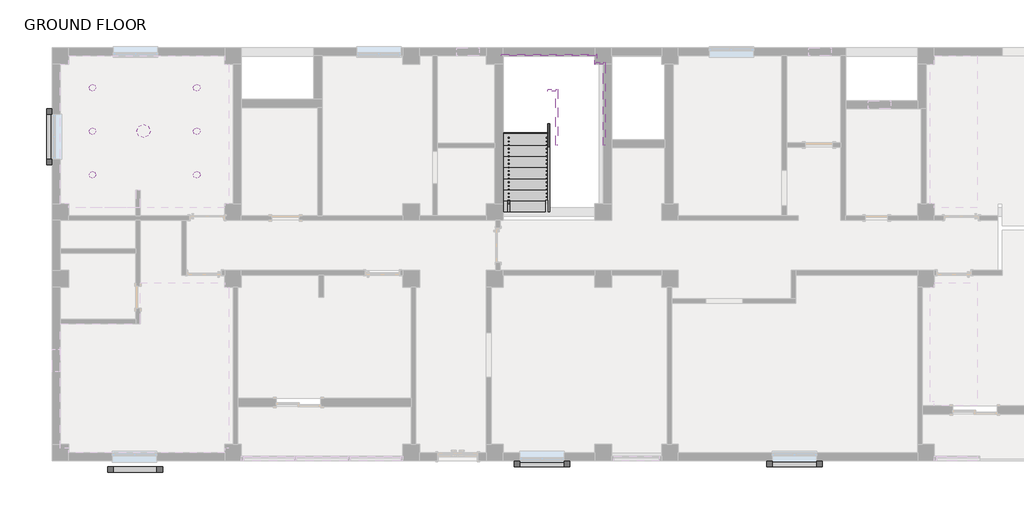
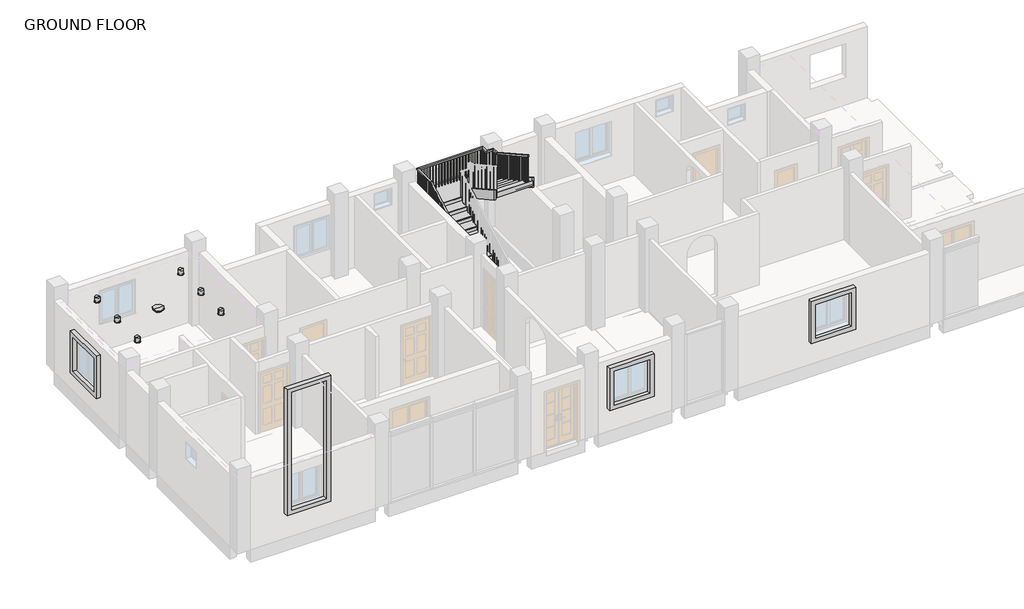
# One storey, part 5 of 5: 8 members, 7 light fixtures, 4 proxies, 1 railing, 1 stair flight.
"""IFC4 building model written with IfcOpenShell, lengths in millimetres."""

from ifc_helpers import new_model, si_unit, frame, origin, place, context, project, spatial, polyline, outline, extrude, faceted_brep, transform, mapped, element, save
from components import generic_models_17_generic_models_17_4194431e, generic_models_21_generic_models_21_07dc1754, generic_models_2_generic_models_2_798ec4a6, light_modern_pendant_14774_baffle_cc9af11b, light_modern_pendant_14774_baffle_b3430626, round_flush_mount_ceiling_light_fixture_18379_round_flush_30de1430, stair_flight_255c1e55

model = new_model("IFC4")

# Units and contexts
model_context = context("Model", 3, world=origin())
ifc_project = project(units=[si_unit("LENGTHUNIT", "METRE", prefix="MILLI")], contexts=[model_context])

# Site, building, storey
site = spatial("IfcSite", under=ifc_project)
building = spatial("IfcBuilding", under=site)
storey = spatial("IfcBuildingStorey", under=building, Name="GROUND FLOOR", Elevation=304.8)

# Proxies
placement = place(None, origin())
generic_models_17_generic_models_17_shape = generic_models_17_generic_models_17_4194431e(model_context)
element("IfcBuildingElementProxy", 1, Name="Generic Models 20 : Generic Models 17", ObjectType="Generic Models 20 : Generic Models 17", at=placement, inside=storey, context=model_context, shape_type="MappedRepresentation", body=[
    mapped(generic_models_17_generic_models_17_shape, transform((0.0, 0.0, -9144.0), x_axis=(1.0, 0.0, 0.0), y_axis=(0.0, 1.0, 0.0), z_axis=(0.0, 0.0, 1.0))),
])
generic_models_21_generic_models_21_shape = generic_models_21_generic_models_21_07dc1754(model_context)
element("IfcBuildingElementProxy", 2, Name="Generic Models 24 : Generic Models 21", ObjectType="Generic Models 24 : Generic Models 21", at=placement, inside=storey, context=model_context, shape_type="MappedRepresentation", body=[
    mapped(generic_models_21_generic_models_21_shape, transform((0.0, 0.0, -9144.0), x_axis=(1.0, 0.0, 0.0), y_axis=(0.0, 1.0, 0.0), z_axis=(0.0, 0.0, 1.0))),
])
element("IfcBuildingElementProxy", 3, Name="Generic Models 28 : Generic Models 21", ObjectType="Generic Models 28 : Generic Models 21", at=placement, inside=storey, context=model_context, shape_type="MappedRepresentation", body=[
    mapped(generic_models_21_generic_models_21_shape, transform((-6905.3372689, 0.0, -9144.0), x_axis=(1.0, 0.0, 0.0), y_axis=(0.0, 1.0, 0.0), z_axis=(0.0, 0.0, 1.0))),
])
generic_models_2_generic_models_2_shape = generic_models_2_generic_models_2_798ec4a6(model_context)
element("IfcBuildingElementProxy", 4, Name="Generic Models 3 : Generic Models 2", ObjectType="Generic Models 3 : Generic Models 2", at=placement, inside=storey, context=model_context, shape_type="MappedRepresentation", body=[
    mapped(generic_models_2_generic_models_2_shape, transform((0.0, 0.0, -6096.0), x_axis=(1.0, 0.0, 0.0), y_axis=(0.0, 1.0, 0.0), z_axis=(0.0, 0.0, 1.0))),
])

# Light fixtures
light_modern_pendant_14774_baffle_shape = light_modern_pendant_14774_baffle_cc9af11b(model_context)
element("IfcLightFixture", 5, ObjectType="LIGHT_-_MODERN_PENDANT_14774 : Baffle", at=placement, inside=storey, context=model_context, shape_type="MappedRepresentation", body=[
    mapped(light_modern_pendant_14774_baffle_shape, transform((-14269.0456086, -897.3794704, 431.8), x_axis=(1.0, 0.0, 0.0), y_axis=(0.0, 1.0, 0.0), z_axis=(0.0, 0.0, 1.0))),
])
element("IfcLightFixture", 6, ObjectType="LIGHT_-_MODERN_PENDANT_14774 : Baffle", at=placement, inside=storey, context=model_context, shape_type="MappedRepresentation", body=[
    mapped(light_modern_pendant_14774_baffle_shape, transform((-14269.0456086, -3284.9794704, 431.8), x_axis=(1.0, 0.0, 0.0), y_axis=(0.0, 1.0, 0.0), z_axis=(0.0, 0.0, 1.0))),
])
element("IfcLightFixture", 7, ObjectType="LIGHT_-_MODERN_PENDANT_14774 : Baffle", at=placement, inside=storey, context=model_context, shape_type="MappedRepresentation", body=[
    mapped(light_modern_pendant_14774_baffle_shape, transform((-14269.0456086, -2091.1794704, 431.8), x_axis=(1.0, 0.0, 0.0), y_axis=(0.0, 1.0, 0.0), z_axis=(0.0, 0.0, 1.0))),
])
light_modern_pendant_14774_baffle_2_shape = light_modern_pendant_14774_baffle_b3430626(model_context)
element("IfcLightFixture", 8, ObjectType="LIGHT_-_MODERN_PENDANT_14774 : Baffle", at=placement, inside=storey, context=model_context, shape_type="MappedRepresentation", body=[
    mapped(light_modern_pendant_14774_baffle_2_shape, transform((-11411.5456086, -897.3794704, 431.8), x_axis=(-1.0, 0.0, 0.0), y_axis=(0.0, -1.0, 0.0), z_axis=(0.0, 0.0, 1.0))),
])
element("IfcLightFixture", 9, ObjectType="LIGHT_-_MODERN_PENDANT_14774 : Baffle", at=placement, inside=storey, context=model_context, shape_type="MappedRepresentation", body=[
    mapped(light_modern_pendant_14774_baffle_2_shape, transform((-11411.5456086, -3284.9794704, 431.8), x_axis=(-1.0, 0.0, 0.0), y_axis=(0.0, -1.0, 0.0), z_axis=(0.0, 0.0, 1.0))),
])
element("IfcLightFixture", 10, ObjectType="LIGHT_-_MODERN_PENDANT_14774 : Baffle", at=placement, inside=storey, context=model_context, shape_type="MappedRepresentation", body=[
    mapped(light_modern_pendant_14774_baffle_2_shape, transform((-11411.5456086, -2091.1794704, 431.8), x_axis=(-1.0, 0.0, 0.0), y_axis=(0.0, -1.0, 0.0), z_axis=(0.0, 0.0, 1.0))),
])
round_flush_mount_ceiling_light_fixture_18379_round_flush_shape = round_flush_mount_ceiling_light_fixture_18379_round_flush_30de1430(model_context)
element("IfcLightFixture", 11, ObjectType="ROUND_FLUSH_MOUNT_CEILING_LIGHT_FIXTURE_18379 : ROUND FLUSH MOUNT CEILING LIGHT FIXTURE", at=placement, inside=storey, context=model_context, shape_type="MappedRepresentation", body=[
    mapped(round_flush_mount_ceiling_light_fixture_18379_round_flush_shape, transform((-12870.8401855, -2091.1794704, 431.8), x_axis=(1.0, 0.0, 0.0), y_axis=(0.0, 1.0, 0.0), z_axis=(0.0, 0.0, 1.0))),
])

# Members
element("IfcMember", 12, ObjectType="Stringer - 2\" Width", at=placement, inside=storey, context=model_context, shape_type="SweptSolid", body=[
    extrude(outline(polyline([(-4300.9794704, 304.8), (-4300.9794704, 512.3983948), (-879.896581, 2413.0), (-252.2749676, 2413.0), (-4047.0349676, 304.8), (-4300.9794704, 304.8)])), frame((-3080.3456086, 0.0, 0.0), z_axis=(1.0, 0.0, 0.0), x_axis=(0.0, 1.0, 0.0)), (0.0, 0.0, 1.0), 50.8),
])
element("IfcMember", 13, ObjectType="Stringer - 2\" Width", at=placement, inside=storey, context=model_context, shape_type="SweptSolid", body=[
    extrude(outline(polyline([(-3080.3456086, -33.7794704), (-3080.3456086, 17.0205296), (-467.6083398, 17.0205296), (-518.4083398, -33.7794704), (-3080.3456086, -33.7794704)])), frame((0.0, 0.0, 2108.2), z_axis=(0.0, 0.0, 1.0), x_axis=(1.0, 0.0, 0.0)), (0.0, 0.0, 1.0), 304.8),
])
element("IfcMember", 14, ObjectType="Stringer - 2\" Width", at=placement, inside=storey, context=model_context, shape_type="SweptSolid", body=[
    extrude(outline(polyline([(-518.4083398, -33.7794704), (-467.6083398, 17.0205296), (-467.6083398, -211.5794704), (-518.4083398, -262.3794704), (-518.4083398, -33.7794704)])), frame((0.0, 0.0, 2108.2), z_axis=(0.0, 0.0, 1.0), x_axis=(1.0, 0.0, 0.0)), (0.0, 0.0, 1.0), 304.8),
])
element("IfcMember", 15, ObjectType="Stringer - 2\" Width", at=placement, inside=storey, context=model_context, shape_type="SweptSolid", body=[
    extrude(outline(polyline([(-518.4083398, -262.3794704), (-467.6083398, -211.5794704), (-289.8083398, -211.5794704), (-289.8083398, -262.3794704), (-518.4083398, -262.3794704)])), frame((0.0, 0.0, 2108.2), z_axis=(0.0, 0.0, 1.0), x_axis=(1.0, 0.0, 0.0)), (0.0, 0.0, 1.0), 304.8),
])
element("IfcMember", 16, ObjectType="Stringer - 2\" Width", at=placement, inside=storey, context=model_context, shape_type="SweptSolid", body=[
    extrude(outline(polyline([(-211.5794704, 2135.1761726), (-211.5794704, 2108.2), (-790.6439732, 2108.2), (-2472.1794704, 3042.3863873), (-2472.1794704, 3391.0650614), (-211.5794704, 2135.1761726)])), frame((-289.8083398, 0.0, 0.0), z_axis=(1.0, 0.0, 0.0), x_axis=(0.0, 1.0, 0.0)), (0.0, 0.0, 1.0), 50.8),
])
element("IfcMember", 17, ObjectType="Stringer - 2\" Width", at=placement, inside=storey, context=model_context, shape_type="SweptSolid", body=[
    extrude(outline(polyline([(-4300.9794704, 304.8), (-4300.9794704, 512.3983948), (-998.9794704, 2346.8428392), (-998.9794704, 1998.1641651), (-4047.0349676, 304.8), (-4300.9794704, 304.8)])), frame((-1810.3456086, 0.0, 0.0), z_axis=(1.0, 0.0, 0.0), x_axis=(0.0, 1.0, 0.0)), (0.0, 0.0, 1.0), 50.8),
])
element("IfcMember", 18, ObjectType="Stringer - 2\" Width", at=placement, inside=storey, context=model_context, shape_type="SweptSolid", body=[
    extrude(outline(polyline([(-1810.3456086, -998.9794704), (-1810.3456086, -948.1794704), (-1585.2083398, -948.1794704), (-1585.2083398, -998.9794704), (-1810.3456086, -998.9794704)])), frame((0.0, 0.0, 2108.2), z_axis=(0.0, 0.0, 1.0), x_axis=(1.0, 0.0, 0.0)), (0.0, 0.0, 1.0), 304.8),
])
element("IfcMember", 19, ObjectType="Stringer - 2\" Width", at=placement, inside=storey, context=model_context, shape_type="SweptSolid", body=[
    extrude(outline(polyline([(-948.1794704, 2544.3983948), (-948.1794704, 2195.7197207), (-2472.1794704, 3042.3863873), (-2472.1794704, 3391.0650614), (-948.1794704, 2544.3983948)])), frame((-1585.2083398, 0.0, 0.0), z_axis=(1.0, 0.0, 0.0), x_axis=(0.0, 1.0, 0.0)), (0.0, 0.0, 1.0), 50.8),
])

# Railing
element("IfcRailing", 20, ObjectType="Handrail - Rectangular", at=placement, inside=storey, context=model_context, shape_type="SolidModel", body=[
    faceted_brep([(-2902.5456086, -4300.9794704, 1388.5333333), (-2902.5456086, -4300.9794704, 1330.420221), (-2851.7456086, -4300.9794704, 1330.420221), (-2851.7456086, -4300.9794704, 1388.5333333), (-2902.5456086, -948.1794704, 3251.2), (-2902.5456086, -935.0158682, 3200.4), (-2851.7456086, -935.0158682, 3200.4), (-2851.7456086, -948.1794704, 3251.2), (-2902.5456086, -160.7794704, 3251.2), (-2902.5456086, -160.7794704, 3200.4), (-2851.7456086, -211.5794704, 3200.4), (-2851.7456086, -211.5794704, 3251.2), (-645.4083398, -160.7794704, 3251.2), (-645.4083398, -160.7794704, 3200.4), (-696.2083398, -211.5794704, 3200.4), (-696.2083398, -211.5794704, 3251.2), (-645.4083398, -389.3794704, 3251.2), (-645.4083398, -389.3794704, 3200.4), (-696.2083398, -440.1794704, 3200.4), (-696.2083398, -440.1794704, 3251.2), (-416.8083398, -389.3794704, 3251.2), (-416.8083398, -389.3794704, 3200.4), (-467.6083398, -440.1794704, 3200.4), (-467.6083398, -440.1794704, 3251.2), (-416.8083398, -643.3794704, 3251.2), (-416.8083398, -656.5430727, 3200.4), (-467.6083398, -656.5430727, 3200.4), (-467.6083398, -643.3794704, 3251.2), (-416.8083398, -2472.1794704, 4267.2), (-467.6083398, -2472.1794704, 4267.2), (-467.6083398, -2472.1794704, 4209.0868876), (-416.8083398, -2472.1794704, 4209.0868876)], [[[0, 1, 2, 3]], [[1, 0, 4, 5]], [[2, 1, 5, 6]], [[3, 2, 6, 7]], [[0, 3, 7, 4]], [[5, 4, 8, 9]], [[6, 5, 9, 10]], [[7, 6, 10, 11]], [[4, 7, 11, 8]], [[9, 8, 12, 13]], [[10, 9, 13, 14]], [[11, 10, 14, 15]], [[8, 11, 15, 12]], [[13, 12, 16, 17]], [[14, 13, 17, 18]], [[15, 14, 18, 19]], [[12, 15, 19, 16]], [[17, 16, 20, 21]], [[18, 17, 21, 22]], [[19, 18, 22, 23]], [[16, 19, 23, 20]], [[21, 20, 24, 25]], [[22, 21, 25, 26]], [[23, 22, 26, 27]], [[20, 23, 27, 24]], [[28, 29, 30, 31]], [[25, 24, 28, 31]], [[26, 25, 31, 30]], [[27, 26, 30, 29]], [[24, 27, 29, 28]]]),
    extrude(outline(polyline([(-2437.2544704, 4189.6841099), (-2437.2544704, 3183.4666667), (-2456.3044704, 3183.4666667), (-2456.3044704, 4200.2674432), (-2437.2544704, 4189.6841099)])), frame((-451.7333398, 0.0, 0.0), z_axis=(1.0, 0.0, 0.0), x_axis=(0.0, 1.0, 0.0)), (0.0, 0.0, 1.0), 19.05),
    extrude(outline(polyline([(-2335.6544704, 4133.2396654), (-2335.6544704, 3183.4666667), (-2354.7044704, 3183.4666667), (-2354.7044704, 4143.8229988), (-2335.6544704, 4133.2396654)])), frame((-451.7333398, 0.0, 0.0), z_axis=(1.0, 0.0, 0.0), x_axis=(0.0, 1.0, 0.0)), (0.0, 0.0, 1.0), 19.05),
    extrude(outline(polyline([(-2234.0544704, 4076.795221), (-2234.0544704, 3183.4666667), (-2253.1044704, 3183.4666667), (-2253.1044704, 4087.3785543), (-2234.0544704, 4076.795221)])), frame((-451.7333398, 0.0, 0.0), z_axis=(1.0, 0.0, 0.0), x_axis=(0.0, 1.0, 0.0)), (0.0, 0.0, 1.0), 19.05),
    extrude(outline(polyline([(-2132.4544704, 4020.3507765), (-2132.4544704, 3014.1333333), (-2151.5044704, 3014.1333333), (-2151.5044704, 4030.9341099), (-2132.4544704, 4020.3507765)])), frame((-451.7333398, 0.0, 0.0), z_axis=(1.0, 0.0, 0.0), x_axis=(0.0, 1.0, 0.0)), (0.0, 0.0, 1.0), 19.05),
    extrude(outline(polyline([(-2030.8544704, 3963.9063321), (-2030.8544704, 3014.1333333), (-2049.9044704, 3014.1333333), (-2049.9044704, 3974.4896654), (-2030.8544704, 3963.9063321)])), frame((-451.7333398, 0.0, 0.0), z_axis=(1.0, 0.0, 0.0), x_axis=(0.0, 1.0, 0.0)), (0.0, 0.0, 1.0), 19.05),
    extrude(outline(polyline([(-1929.2544704, 3907.4618876), (-1929.2544704, 3014.1333333), (-1948.3044704, 3014.1333333), (-1948.3044704, 3918.045221), (-1929.2544704, 3907.4618876)])), frame((-451.7333398, 0.0, 0.0), z_axis=(1.0, 0.0, 0.0), x_axis=(0.0, 1.0, 0.0)), (0.0, 0.0, 1.0), 19.05),
    extrude(outline(polyline([(-1827.6544704, 3851.0174432), (-1827.6544704, 2844.8), (-1846.7044704, 2844.8), (-1846.7044704, 3861.6007765), (-1827.6544704, 3851.0174432)])), frame((-451.7333398, 0.0, 0.0), z_axis=(1.0, 0.0, 0.0), x_axis=(0.0, 1.0, 0.0)), (0.0, 0.0, 1.0), 19.05),
    extrude(outline(polyline([(-1726.0544704, 3794.5729988), (-1726.0544704, 2844.8), (-1745.1044704, 2844.8), (-1745.1044704, 3805.1563321), (-1726.0544704, 3794.5729988)])), frame((-451.7333398, 0.0, 0.0), z_axis=(1.0, 0.0, 0.0), x_axis=(0.0, 1.0, 0.0)), (0.0, 0.0, 1.0), 19.05),
    extrude(outline(polyline([(-1624.4544704, 3738.1285543), (-1624.4544704, 2844.8), (-1643.5044704, 2844.8), (-1643.5044704, 3748.7118876), (-1624.4544704, 3738.1285543)])), frame((-451.7333398, 0.0, 0.0), z_axis=(1.0, 0.0, 0.0), x_axis=(0.0, 1.0, 0.0)), (0.0, 0.0, 1.0), 19.05),
    extrude(outline(polyline([(-1522.8544704, 3681.6841099), (-1522.8544704, 2675.4666667), (-1541.9044704, 2675.4666667), (-1541.9044704, 3692.2674432), (-1522.8544704, 3681.6841099)])), frame((-451.7333398, 0.0, 0.0), z_axis=(1.0, 0.0, 0.0), x_axis=(0.0, 1.0, 0.0)), (0.0, 0.0, 1.0), 19.05),
    extrude(outline(polyline([(-1421.2544704, 3625.2396654), (-1421.2544704, 2675.4666667), (-1440.3044704, 2675.4666667), (-1440.3044704, 3635.8229988), (-1421.2544704, 3625.2396654)])), frame((-451.7333398, 0.0, 0.0), z_axis=(1.0, 0.0, 0.0), x_axis=(0.0, 1.0, 0.0)), (0.0, 0.0, 1.0), 19.05),
    extrude(outline(polyline([(-1319.6544704, 3568.795221), (-1319.6544704, 2675.4666667), (-1338.7044704, 2675.4666667), (-1338.7044704, 3579.3785543), (-1319.6544704, 3568.795221)])), frame((-451.7333398, 0.0, 0.0), z_axis=(1.0, 0.0, 0.0), x_axis=(0.0, 1.0, 0.0)), (0.0, 0.0, 1.0), 19.05),
    extrude(outline(polyline([(-1218.0544704, 3512.3507765), (-1218.0544704, 2506.1333333), (-1237.1044704, 2506.1333333), (-1237.1044704, 3522.9341099), (-1218.0544704, 3512.3507765)])), frame((-451.7333398, 0.0, 0.0), z_axis=(1.0, 0.0, 0.0), x_axis=(0.0, 1.0, 0.0)), (0.0, 0.0, 1.0), 19.05),
    extrude(outline(polyline([(-1116.4544704, 3455.9063321), (-1116.4544704, 2506.1333333), (-1135.5044704, 2506.1333333), (-1135.5044704, 3466.4896654), (-1116.4544704, 3455.9063321)])), frame((-451.7333398, 0.0, 0.0), z_axis=(1.0, 0.0, 0.0), x_axis=(0.0, 1.0, 0.0)), (0.0, 0.0, 1.0), 19.05),
    extrude(outline(polyline([(-1014.8544704, 3399.4618876), (-1014.8544704, 2506.1333333), (-1033.9044704, 2506.1333333), (-1033.9044704, 3410.045221), (-1014.8544704, 3399.4618876)])), frame((-451.7333398, 0.0, 0.0), z_axis=(1.0, 0.0, 0.0), x_axis=(0.0, 1.0, 0.0)), (0.0, 0.0, 1.0), 19.05),
    extrude(outline(polyline([(-913.2544704, 3343.0174432), (-913.2544704, 2336.8), (-932.3044704, 2336.8), (-932.3044704, 3353.6007765), (-913.2544704, 3343.0174432)])), frame((-451.7333398, 0.0, 0.0), z_axis=(1.0, 0.0, 0.0), x_axis=(0.0, 1.0, 0.0)), (0.0, 0.0, 1.0), 19.05),
    extrude(outline(polyline([(-811.6544704, 3286.5729988), (-811.6544704, 2336.8), (-830.7044704, 2336.8), (-830.7044704, 3297.1563321), (-811.6544704, 3286.5729988)])), frame((-451.7333398, 0.0, 0.0), z_axis=(1.0, 0.0, 0.0), x_axis=(0.0, 1.0, 0.0)), (0.0, 0.0, 1.0), 19.05),
    extrude(outline(polyline([(-710.0544704, 3230.1285543), (-710.0544704, 2336.8), (-729.1044704, 2336.8), (-729.1044704, 3240.7118876), (-710.0544704, 3230.1285543)])), frame((-451.7333398, 0.0, 0.0), z_axis=(1.0, 0.0, 0.0), x_axis=(0.0, 1.0, 0.0)), (0.0, 0.0, 1.0), 19.05),
    extrude(outline(polyline([(-432.6833398, -608.4544704), (-432.6833398, -627.5044704), (-451.7333398, -627.5044704), (-451.7333398, -608.4544704), (-432.6833398, -608.4544704)])), frame((0.0, 0.0, 2336.8), z_axis=(0.0, 0.0, 1.0), x_axis=(1.0, 0.0, 0.0)), (0.0, 0.0, 1.0), 863.6),
    extrude(outline(polyline([(-432.6833398, -506.8544704), (-432.6833398, -525.9044704), (-451.7333398, -525.9044704), (-451.7333398, -506.8544704), (-432.6833398, -506.8544704)])), frame((0.0, 0.0, 2336.8), z_axis=(0.0, 0.0, 1.0), x_axis=(1.0, 0.0, 0.0)), (0.0, 0.0, 1.0), 863.6),
    extrude(outline(polyline([(-477.1333398, -405.2544704), (-458.0833398, -405.2544704), (-458.0833398, -424.3044704), (-477.1333398, -424.3044704), (-477.1333398, -405.2544704)])), frame((0.0, 0.0, 2336.8), z_axis=(0.0, 0.0, 1.0), x_axis=(1.0, 0.0, 0.0)), (0.0, 0.0, 1.0), 863.6),
    extrude(outline(polyline([(-578.7333398, -405.2544704), (-559.6833398, -405.2544704), (-559.6833398, -424.3044704), (-578.7333398, -424.3044704), (-578.7333398, -405.2544704)])), frame((0.0, 0.0, 2336.8), z_axis=(0.0, 0.0, 1.0), x_axis=(1.0, 0.0, 0.0)), (0.0, 0.0, 1.0), 863.6),
    extrude(outline(polyline([(-661.2833398, -379.8544704), (-661.2833398, -398.9044704), (-680.3333398, -398.9044704), (-680.3333398, -379.8544704), (-661.2833398, -379.8544704)])), frame((0.0, 0.0, 2336.8), z_axis=(0.0, 0.0, 1.0), x_axis=(1.0, 0.0, 0.0)), (0.0, 0.0, 1.0), 863.6),
    extrude(outline(polyline([(-661.2833398, -278.2544704), (-661.2833398, -297.3044704), (-680.3333398, -297.3044704), (-680.3333398, -278.2544704), (-661.2833398, -278.2544704)])), frame((0.0, 0.0, 2336.8), z_axis=(0.0, 0.0, 1.0), x_axis=(1.0, 0.0, 0.0)), (0.0, 0.0, 1.0), 863.6),
    extrude(outline(polyline([(-753.0706086, -176.6544704), (-734.0206086, -176.6544704), (-734.0206086, -195.7044704), (-753.0706086, -195.7044704), (-753.0706086, -176.6544704)])), frame((0.0, 0.0, 2336.8), z_axis=(0.0, 0.0, 1.0), x_axis=(1.0, 0.0, 0.0)), (0.0, 0.0, 1.0), 863.6),
    extrude(outline(polyline([(-854.6706086, -176.6544704), (-835.6206086, -176.6544704), (-835.6206086, -195.7044704), (-854.6706086, -195.7044704), (-854.6706086, -176.6544704)])), frame((0.0, 0.0, 2336.8), z_axis=(0.0, 0.0, 1.0), x_axis=(1.0, 0.0, 0.0)), (0.0, 0.0, 1.0), 863.6),
    extrude(outline(polyline([(-956.2706086, -176.6544704), (-937.2206086, -176.6544704), (-937.2206086, -195.7044704), (-956.2706086, -195.7044704), (-956.2706086, -176.6544704)])), frame((0.0, 0.0, 2336.8), z_axis=(0.0, 0.0, 1.0), x_axis=(1.0, 0.0, 0.0)), (0.0, 0.0, 1.0), 863.6),
    extrude(outline(polyline([(-1057.8706086, -176.6544704), (-1038.8206086, -176.6544704), (-1038.8206086, -195.7044704), (-1057.8706086, -195.7044704), (-1057.8706086, -176.6544704)])), frame((0.0, 0.0, 2336.8), z_axis=(0.0, 0.0, 1.0), x_axis=(1.0, 0.0, 0.0)), (0.0, 0.0, 1.0), 863.6),
    extrude(outline(polyline([(-1159.4706086, -176.6544704), (-1140.4206086, -176.6544704), (-1140.4206086, -195.7044704), (-1159.4706086, -195.7044704), (-1159.4706086, -176.6544704)])), frame((0.0, 0.0, 2336.8), z_axis=(0.0, 0.0, 1.0), x_axis=(1.0, 0.0, 0.0)), (0.0, 0.0, 1.0), 863.6),
    extrude(outline(polyline([(-1261.0706086, -176.6544704), (-1242.0206086, -176.6544704), (-1242.0206086, -195.7044704), (-1261.0706086, -195.7044704), (-1261.0706086, -176.6544704)])), frame((0.0, 0.0, 2336.8), z_axis=(0.0, 0.0, 1.0), x_axis=(1.0, 0.0, 0.0)), (0.0, 0.0, 1.0), 863.6),
    extrude(outline(polyline([(-1362.6706086, -176.6544704), (-1343.6206086, -176.6544704), (-1343.6206086, -195.7044704), (-1362.6706086, -195.7044704), (-1362.6706086, -176.6544704)])), frame((0.0, 0.0, 2336.8), z_axis=(0.0, 0.0, 1.0), x_axis=(1.0, 0.0, 0.0)), (0.0, 0.0, 1.0), 863.6),
    extrude(outline(polyline([(-1464.2706086, -176.6544704), (-1445.2206086, -176.6544704), (-1445.2206086, -195.7044704), (-1464.2706086, -195.7044704), (-1464.2706086, -176.6544704)])), frame((0.0, 0.0, 2336.8), z_axis=(0.0, 0.0, 1.0), x_axis=(1.0, 0.0, 0.0)), (0.0, 0.0, 1.0), 863.6),
    extrude(outline(polyline([(-1565.8706086, -176.6544704), (-1546.8206086, -176.6544704), (-1546.8206086, -195.7044704), (-1565.8706086, -195.7044704), (-1565.8706086, -176.6544704)])), frame((0.0, 0.0, 2336.8), z_axis=(0.0, 0.0, 1.0), x_axis=(1.0, 0.0, 0.0)), (0.0, 0.0, 1.0), 863.6),
    extrude(outline(polyline([(-1667.4706086, -176.6544704), (-1648.4206086, -176.6544704), (-1648.4206086, -195.7044704), (-1667.4706086, -195.7044704), (-1667.4706086, -176.6544704)])), frame((0.0, 0.0, 2336.8), z_axis=(0.0, 0.0, 1.0), x_axis=(1.0, 0.0, 0.0)), (0.0, 0.0, 1.0), 863.6),
    extrude(outline(polyline([(-1769.0706086, -176.6544704), (-1750.0206086, -176.6544704), (-1750.0206086, -195.7044704), (-1769.0706086, -195.7044704), (-1769.0706086, -176.6544704)])), frame((0.0, 0.0, 2336.8), z_axis=(0.0, 0.0, 1.0), x_axis=(1.0, 0.0, 0.0)), (0.0, 0.0, 1.0), 863.6),
    extrude(outline(polyline([(-1870.6706086, -176.6544704), (-1851.6206086, -176.6544704), (-1851.6206086, -195.7044704), (-1870.6706086, -195.7044704), (-1870.6706086, -176.6544704)])), frame((0.0, 0.0, 2336.8), z_axis=(0.0, 0.0, 1.0), x_axis=(1.0, 0.0, 0.0)), (0.0, 0.0, 1.0), 863.6),
    extrude(outline(polyline([(-1972.2706086, -176.6544704), (-1953.2206086, -176.6544704), (-1953.2206086, -195.7044704), (-1972.2706086, -195.7044704), (-1972.2706086, -176.6544704)])), frame((0.0, 0.0, 2336.8), z_axis=(0.0, 0.0, 1.0), x_axis=(1.0, 0.0, 0.0)), (0.0, 0.0, 1.0), 863.6),
    extrude(outline(polyline([(-2073.8706086, -176.6544704), (-2054.8206086, -176.6544704), (-2054.8206086, -195.7044704), (-2073.8706086, -195.7044704), (-2073.8706086, -176.6544704)])), frame((0.0, 0.0, 2336.8), z_axis=(0.0, 0.0, 1.0), x_axis=(1.0, 0.0, 0.0)), (0.0, 0.0, 1.0), 863.6),
    extrude(outline(polyline([(-2175.4706086, -176.6544704), (-2156.4206086, -176.6544704), (-2156.4206086, -195.7044704), (-2175.4706086, -195.7044704), (-2175.4706086, -176.6544704)])), frame((0.0, 0.0, 2336.8), z_axis=(0.0, 0.0, 1.0), x_axis=(1.0, 0.0, 0.0)), (0.0, 0.0, 1.0), 863.6),
    extrude(outline(polyline([(-2277.0706086, -176.6544704), (-2258.0206086, -176.6544704), (-2258.0206086, -195.7044704), (-2277.0706086, -195.7044704), (-2277.0706086, -176.6544704)])), frame((0.0, 0.0, 2336.8), z_axis=(0.0, 0.0, 1.0), x_axis=(1.0, 0.0, 0.0)), (0.0, 0.0, 1.0), 863.6),
    extrude(outline(polyline([(-2378.6706086, -176.6544704), (-2359.6206086, -176.6544704), (-2359.6206086, -195.7044704), (-2378.6706086, -195.7044704), (-2378.6706086, -176.6544704)])), frame((0.0, 0.0, 2336.8), z_axis=(0.0, 0.0, 1.0), x_axis=(1.0, 0.0, 0.0)), (0.0, 0.0, 1.0), 863.6),
    extrude(outline(polyline([(-2480.2706086, -176.6544704), (-2461.2206086, -176.6544704), (-2461.2206086, -195.7044704), (-2480.2706086, -195.7044704), (-2480.2706086, -176.6544704)])), frame((0.0, 0.0, 2336.8), z_axis=(0.0, 0.0, 1.0), x_axis=(1.0, 0.0, 0.0)), (0.0, 0.0, 1.0), 863.6),
    extrude(outline(polyline([(-2581.8706086, -176.6544704), (-2562.8206086, -176.6544704), (-2562.8206086, -195.7044704), (-2581.8706086, -195.7044704), (-2581.8706086, -176.6544704)])), frame((0.0, 0.0, 2336.8), z_axis=(0.0, 0.0, 1.0), x_axis=(1.0, 0.0, 0.0)), (0.0, 0.0, 1.0), 863.6),
    extrude(outline(polyline([(-2683.4706086, -176.6544704), (-2664.4206086, -176.6544704), (-2664.4206086, -195.7044704), (-2683.4706086, -195.7044704), (-2683.4706086, -176.6544704)])), frame((0.0, 0.0, 2336.8), z_axis=(0.0, 0.0, 1.0), x_axis=(1.0, 0.0, 0.0)), (0.0, 0.0, 1.0), 863.6),
    extrude(outline(polyline([(-2785.0706086, -176.6544704), (-2766.0206086, -176.6544704), (-2766.0206086, -195.7044704), (-2785.0706086, -195.7044704), (-2785.0706086, -176.6544704)])), frame((0.0, 0.0, 2336.8), z_axis=(0.0, 0.0, 1.0), x_axis=(1.0, 0.0, 0.0)), (0.0, 0.0, 1.0), 863.6),
    extrude(outline(polyline([(-2886.6706086, -246.5044704), (-2886.6706086, -227.4544704), (-2867.6206086, -227.4544704), (-2867.6206086, -246.5044704), (-2886.6706086, -246.5044704)])), frame((0.0, 0.0, 2336.8), z_axis=(0.0, 0.0, 1.0), x_axis=(1.0, 0.0, 0.0)), (0.0, 0.0, 1.0), 863.6),
    extrude(outline(polyline([(-2886.6706086, -348.1044704), (-2886.6706086, -329.0544704), (-2867.6206086, -329.0544704), (-2867.6206086, -348.1044704), (-2886.6706086, -348.1044704)])), frame((0.0, 0.0, 2336.8), z_axis=(0.0, 0.0, 1.0), x_axis=(1.0, 0.0, 0.0)), (0.0, 0.0, 1.0), 863.6),
    extrude(outline(polyline([(-2886.6706086, -449.7044704), (-2886.6706086, -430.6544704), (-2867.6206086, -430.6544704), (-2867.6206086, -449.7044704), (-2886.6706086, -449.7044704)])), frame((0.0, 0.0, 2336.8), z_axis=(0.0, 0.0, 1.0), x_axis=(1.0, 0.0, 0.0)), (0.0, 0.0, 1.0), 863.6),
    extrude(outline(polyline([(-2886.6706086, -551.3044704), (-2886.6706086, -532.2544704), (-2867.6206086, -532.2544704), (-2867.6206086, -551.3044704), (-2886.6706086, -551.3044704)])), frame((0.0, 0.0, 2336.8), z_axis=(0.0, 0.0, 1.0), x_axis=(1.0, 0.0, 0.0)), (0.0, 0.0, 1.0), 863.6),
    extrude(outline(polyline([(-2886.6706086, -652.9044704), (-2886.6706086, -633.8544704), (-2867.6206086, -633.8544704), (-2867.6206086, -652.9044704), (-2886.6706086, -652.9044704)])), frame((0.0, 0.0, 2336.8), z_axis=(0.0, 0.0, 1.0), x_axis=(1.0, 0.0, 0.0)), (0.0, 0.0, 1.0), 863.6),
    extrude(outline(polyline([(-2886.6706086, -754.5044704), (-2886.6706086, -735.4544704), (-2867.6206086, -735.4544704), (-2867.6206086, -754.5044704), (-2886.6706086, -754.5044704)])), frame((0.0, 0.0, 2336.8), z_axis=(0.0, 0.0, 1.0), x_axis=(1.0, 0.0, 0.0)), (0.0, 0.0, 1.0), 863.6),
    extrude(outline(polyline([(-2886.6706086, -856.1044704), (-2886.6706086, -837.0544704), (-2867.6206086, -837.0544704), (-2867.6206086, -856.1044704), (-2886.6706086, -856.1044704)])), frame((0.0, 0.0, 2336.8), z_axis=(0.0, 0.0, 1.0), x_axis=(1.0, 0.0, 0.0)), (0.0, 0.0, 1.0), 863.6),
    extrude(outline(polyline([(-938.6544704, 3198.3785543), (-938.6544704, 2336.8), (-957.7044704, 2336.8), (-957.7044704, 3187.795221), (-938.6544704, 3198.3785543)])), frame((-2886.6706086, 0.0, 0.0), z_axis=(1.0, 0.0, 0.0), x_axis=(0.0, 1.0, 0.0)), (0.0, 0.0, 1.0), 19.05),
    extrude(outline(polyline([(-1040.2544704, 3141.9341099), (-1040.2544704, 2167.4666667), (-1059.3044704, 2167.4666667), (-1059.3044704, 3131.3507765), (-1040.2544704, 3141.9341099)])), frame((-2886.6706086, 0.0, 0.0), z_axis=(1.0, 0.0, 0.0), x_axis=(0.0, 1.0, 0.0)), (0.0, 0.0, 1.0), 19.05),
    extrude(outline(polyline([(-1141.8544704, 3085.4896654), (-1141.8544704, 2167.4666667), (-1160.9044704, 2167.4666667), (-1160.9044704, 3074.9063321), (-1141.8544704, 3085.4896654)])), frame((-2886.6706086, 0.0, 0.0), z_axis=(1.0, 0.0, 0.0), x_axis=(0.0, 1.0, 0.0)), (0.0, 0.0, 1.0), 19.05),
    extrude(outline(polyline([(-1243.4544704, 3029.045221), (-1243.4544704, 2167.4666667), (-1262.5044704, 2167.4666667), (-1262.5044704, 3018.4618876), (-1243.4544704, 3029.045221)])), frame((-2886.6706086, 0.0, 0.0), z_axis=(1.0, 0.0, 0.0), x_axis=(0.0, 1.0, 0.0)), (0.0, 0.0, 1.0), 19.05),
    extrude(outline(polyline([(-1345.0544704, 2972.6007765), (-1345.0544704, 1998.1333333), (-1364.1044704, 1998.1333333), (-1364.1044704, 2962.0174432), (-1345.0544704, 2972.6007765)])), frame((-2886.6706086, 0.0, 0.0), z_axis=(1.0, 0.0, 0.0), x_axis=(0.0, 1.0, 0.0)), (0.0, 0.0, 1.0), 19.05),
    extrude(outline(polyline([(-1446.6544704, 2916.1563321), (-1446.6544704, 1998.1333333), (-1465.7044704, 1998.1333333), (-1465.7044704, 2905.5729988), (-1446.6544704, 2916.1563321)])), frame((-2886.6706086, 0.0, 0.0), z_axis=(1.0, 0.0, 0.0), x_axis=(0.0, 1.0, 0.0)), (0.0, 0.0, 1.0), 19.05),
    extrude(outline(polyline([(-1548.2544704, 2859.7118876), (-1548.2544704, 1998.1333333), (-1567.3044704, 1998.1333333), (-1567.3044704, 2849.1285543), (-1548.2544704, 2859.7118876)])), frame((-2886.6706086, 0.0, 0.0), z_axis=(1.0, 0.0, 0.0), x_axis=(0.0, 1.0, 0.0)), (0.0, 0.0, 1.0), 19.05),
    extrude(outline(polyline([(-1649.8544704, 2803.2674432), (-1649.8544704, 1828.8), (-1668.9044704, 1828.8), (-1668.9044704, 2792.6841099), (-1649.8544704, 2803.2674432)])), frame((-2886.6706086, 0.0, 0.0), z_axis=(1.0, 0.0, 0.0), x_axis=(0.0, 1.0, 0.0)), (0.0, 0.0, 1.0), 19.05),
    extrude(outline(polyline([(-1751.4544704, 2746.8229988), (-1751.4544704, 1828.8), (-1770.5044704, 1828.8), (-1770.5044704, 2736.2396654), (-1751.4544704, 2746.8229988)])), frame((-2886.6706086, 0.0, 0.0), z_axis=(1.0, 0.0, 0.0), x_axis=(0.0, 1.0, 0.0)), (0.0, 0.0, 1.0), 19.05),
    extrude(outline(polyline([(-1853.0544704, 2690.3785543), (-1853.0544704, 1828.8), (-1872.1044704, 1828.8), (-1872.1044704, 2679.795221), (-1853.0544704, 2690.3785543)])), frame((-2886.6706086, 0.0, 0.0), z_axis=(1.0, 0.0, 0.0), x_axis=(0.0, 1.0, 0.0)), (0.0, 0.0, 1.0), 19.05),
    extrude(outline(polyline([(-1954.6544704, 2633.9341099), (-1954.6544704, 1659.4666667), (-1973.7044704, 1659.4666667), (-1973.7044704, 2623.3507765), (-1954.6544704, 2633.9341099)])), frame((-2886.6706086, 0.0, 0.0), z_axis=(1.0, 0.0, 0.0), x_axis=(0.0, 1.0, 0.0)), (0.0, 0.0, 1.0), 19.05),
    extrude(outline(polyline([(-2056.2544704, 2577.4896654), (-2056.2544704, 1659.4666667), (-2075.3044704, 1659.4666667), (-2075.3044704, 2566.9063321), (-2056.2544704, 2577.4896654)])), frame((-2886.6706086, 0.0, 0.0), z_axis=(1.0, 0.0, 0.0), x_axis=(0.0, 1.0, 0.0)), (0.0, 0.0, 1.0), 19.05),
    extrude(outline(polyline([(-2157.8544704, 2521.045221), (-2157.8544704, 1659.4666667), (-2176.9044704, 1659.4666667), (-2176.9044704, 2510.4618876), (-2157.8544704, 2521.045221)])), frame((-2886.6706086, 0.0, 0.0), z_axis=(1.0, 0.0, 0.0), x_axis=(0.0, 1.0, 0.0)), (0.0, 0.0, 1.0), 19.05),
    extrude(outline(polyline([(-2259.4544704, 2464.6007765), (-2259.4544704, 1490.1333333), (-2278.5044704, 1490.1333333), (-2278.5044704, 2454.0174432), (-2259.4544704, 2464.6007765)])), frame((-2886.6706086, 0.0, 0.0), z_axis=(1.0, 0.0, 0.0), x_axis=(0.0, 1.0, 0.0)), (0.0, 0.0, 1.0), 19.05),
    extrude(outline(polyline([(-2361.0544704, 2408.1563321), (-2361.0544704, 1490.1333333), (-2380.1044704, 1490.1333333), (-2380.1044704, 2397.5729988), (-2361.0544704, 2408.1563321)])), frame((-2886.6706086, 0.0, 0.0), z_axis=(1.0, 0.0, 0.0), x_axis=(0.0, 1.0, 0.0)), (0.0, 0.0, 1.0), 19.05),
    extrude(outline(polyline([(-2462.6544704, 2351.7118876), (-2462.6544704, 1490.1333333), (-2481.7044704, 1490.1333333), (-2481.7044704, 2341.1285543), (-2462.6544704, 2351.7118876)])), frame((-2886.6706086, 0.0, 0.0), z_axis=(1.0, 0.0, 0.0), x_axis=(0.0, 1.0, 0.0)), (0.0, 0.0, 1.0), 19.05),
    extrude(outline(polyline([(-2564.2544704, 2295.2674432), (-2564.2544704, 1320.8), (-2583.3044704, 1320.8), (-2583.3044704, 2284.6841099), (-2564.2544704, 2295.2674432)])), frame((-2886.6706086, 0.0, 0.0), z_axis=(1.0, 0.0, 0.0), x_axis=(0.0, 1.0, 0.0)), (0.0, 0.0, 1.0), 19.05),
    extrude(outline(polyline([(-2665.8544704, 2238.8229988), (-2665.8544704, 1320.8), (-2684.9044704, 1320.8), (-2684.9044704, 2228.2396654), (-2665.8544704, 2238.8229988)])), frame((-2886.6706086, 0.0, 0.0), z_axis=(1.0, 0.0, 0.0), x_axis=(0.0, 1.0, 0.0)), (0.0, 0.0, 1.0), 19.05),
    extrude(outline(polyline([(-2767.4544704, 2182.3785543), (-2767.4544704, 1320.8), (-2786.5044704, 1320.8), (-2786.5044704, 2171.795221), (-2767.4544704, 2182.3785543)])), frame((-2886.6706086, 0.0, 0.0), z_axis=(1.0, 0.0, 0.0), x_axis=(0.0, 1.0, 0.0)), (0.0, 0.0, 1.0), 19.05),
    extrude(outline(polyline([(-2869.0544704, 2125.9341099), (-2869.0544704, 1151.4666667), (-2888.1044704, 1151.4666667), (-2888.1044704, 2115.3507765), (-2869.0544704, 2125.9341099)])), frame((-2886.6706086, 0.0, 0.0), z_axis=(1.0, 0.0, 0.0), x_axis=(0.0, 1.0, 0.0)), (0.0, 0.0, 1.0), 19.05),
    extrude(outline(polyline([(-2970.6544704, 2069.4896654), (-2970.6544704, 1151.4666667), (-2989.7044704, 1151.4666667), (-2989.7044704, 2058.9063321), (-2970.6544704, 2069.4896654)])), frame((-2886.6706086, 0.0, 0.0), z_axis=(1.0, 0.0, 0.0), x_axis=(0.0, 1.0, 0.0)), (0.0, 0.0, 1.0), 19.05),
    extrude(outline(polyline([(-3072.2544704, 2013.045221), (-3072.2544704, 1151.4666667), (-3091.3044704, 1151.4666667), (-3091.3044704, 2002.4618876), (-3072.2544704, 2013.045221)])), frame((-2886.6706086, 0.0, 0.0), z_axis=(1.0, 0.0, 0.0), x_axis=(0.0, 1.0, 0.0)), (0.0, 0.0, 1.0), 19.05),
    extrude(outline(polyline([(-3173.8544704, 1956.6007765), (-3173.8544704, 982.1333333), (-3192.9044704, 982.1333333), (-3192.9044704, 1946.0174432), (-3173.8544704, 1956.6007765)])), frame((-2886.6706086, 0.0, 0.0), z_axis=(1.0, 0.0, 0.0), x_axis=(0.0, 1.0, 0.0)), (0.0, 0.0, 1.0), 19.05),
    extrude(outline(polyline([(-3275.4544704, 1900.1563321), (-3275.4544704, 982.1333333), (-3294.5044704, 982.1333333), (-3294.5044704, 1889.5729988), (-3275.4544704, 1900.1563321)])), frame((-2886.6706086, 0.0, 0.0), z_axis=(1.0, 0.0, 0.0), x_axis=(0.0, 1.0, 0.0)), (0.0, 0.0, 1.0), 19.05),
    extrude(outline(polyline([(-3377.0544704, 1843.7118876), (-3377.0544704, 982.1333333), (-3396.1044704, 982.1333333), (-3396.1044704, 1833.1285543), (-3377.0544704, 1843.7118876)])), frame((-2886.6706086, 0.0, 0.0), z_axis=(1.0, 0.0, 0.0), x_axis=(0.0, 1.0, 0.0)), (0.0, 0.0, 1.0), 19.05),
    extrude(outline(polyline([(-3478.6544704, 1787.2674432), (-3478.6544704, 812.8), (-3497.7044704, 812.8), (-3497.7044704, 1776.6841099), (-3478.6544704, 1787.2674432)])), frame((-2886.6706086, 0.0, 0.0), z_axis=(1.0, 0.0, 0.0), x_axis=(0.0, 1.0, 0.0)), (0.0, 0.0, 1.0), 19.05),
    extrude(outline(polyline([(-3580.2544704, 1730.8229988), (-3580.2544704, 812.8), (-3599.3044704, 812.8), (-3599.3044704, 1720.2396654), (-3580.2544704, 1730.8229988)])), frame((-2886.6706086, 0.0, 0.0), z_axis=(1.0, 0.0, 0.0), x_axis=(0.0, 1.0, 0.0)), (0.0, 0.0, 1.0), 19.05),
    extrude(outline(polyline([(-3681.8544704, 1674.3785543), (-3681.8544704, 812.8), (-3700.9044704, 812.8), (-3700.9044704, 1663.795221), (-3681.8544704, 1674.3785543)])), frame((-2886.6706086, 0.0, 0.0), z_axis=(1.0, 0.0, 0.0), x_axis=(0.0, 1.0, 0.0)), (0.0, 0.0, 1.0), 19.05),
    extrude(outline(polyline([(-3783.4544704, 1617.9341099), (-3783.4544704, 643.4666667), (-3802.5044704, 643.4666667), (-3802.5044704, 1607.3507765), (-3783.4544704, 1617.9341099)])), frame((-2886.6706086, 0.0, 0.0), z_axis=(1.0, 0.0, 0.0), x_axis=(0.0, 1.0, 0.0)), (0.0, 0.0, 1.0), 19.05),
    extrude(outline(polyline([(-3885.0544704, 1561.4896654), (-3885.0544704, 643.4666667), (-3904.1044704, 643.4666667), (-3904.1044704, 1550.9063321), (-3885.0544704, 1561.4896654)])), frame((-2886.6706086, 0.0, 0.0), z_axis=(1.0, 0.0, 0.0), x_axis=(0.0, 1.0, 0.0)), (0.0, 0.0, 1.0), 19.05),
    extrude(outline(polyline([(-3986.6544704, 1505.045221), (-3986.6544704, 643.4666667), (-4005.7044704, 643.4666667), (-4005.7044704, 1494.4618876), (-3986.6544704, 1505.045221)])), frame((-2886.6706086, 0.0, 0.0), z_axis=(1.0, 0.0, 0.0), x_axis=(0.0, 1.0, 0.0)), (0.0, 0.0, 1.0), 19.05),
    extrude(outline(polyline([(-4088.2544704, 1448.6007765), (-4088.2544704, 474.1333333), (-4107.3044704, 474.1333333), (-4107.3044704, 1438.0174432), (-4088.2544704, 1448.6007765)])), frame((-2886.6706086, 0.0, 0.0), z_axis=(1.0, 0.0, 0.0), x_axis=(0.0, 1.0, 0.0)), (0.0, 0.0, 1.0), 19.05),
    extrude(outline(polyline([(-4189.8544704, 1392.1563321), (-4189.8544704, 474.1333333), (-4208.9044704, 474.1333333), (-4208.9044704, 1381.5729988), (-4189.8544704, 1392.1563321)])), frame((-2886.6706086, 0.0, 0.0), z_axis=(1.0, 0.0, 0.0), x_axis=(0.0, 1.0, 0.0)), (0.0, 0.0, 1.0), 19.05),
    extrude(outline(polyline([(-451.7333398, -405.2544704), (-432.6833398, -405.2544704), (-432.6833398, -424.3044704), (-451.7333398, -424.3044704), (-451.7333398, -405.2544704)])), frame((0.0, 0.0, 2336.8), z_axis=(0.0, 0.0, 1.0), x_axis=(1.0, 0.0, 0.0)), (0.0, 0.0, 1.0), 863.6),
    extrude(outline(polyline([(-661.2833398, -405.2544704), (-661.2833398, -424.3044704), (-680.3333398, -424.3044704), (-680.3333398, -405.2544704), (-661.2833398, -405.2544704)])), frame((0.0, 0.0, 2336.8), z_axis=(0.0, 0.0, 1.0), x_axis=(1.0, 0.0, 0.0)), (0.0, 0.0, 1.0), 863.6),
    extrude(outline(polyline([(-680.3333398, -176.6544704), (-661.2833398, -176.6544704), (-661.2833398, -195.7044704), (-680.3333398, -195.7044704), (-680.3333398, -176.6544704)])), frame((0.0, 0.0, 2336.8), z_axis=(0.0, 0.0, 1.0), x_axis=(1.0, 0.0, 0.0)), (0.0, 0.0, 1.0), 863.6),
    extrude(outline(polyline([(-2886.6706086, -195.7044704), (-2886.6706086, -176.6544704), (-2867.6206086, -176.6544704), (-2867.6206086, -195.7044704), (-2886.6706086, -195.7044704)])), frame((0.0, 0.0, 2336.8), z_axis=(0.0, 0.0, 1.0), x_axis=(1.0, 0.0, 0.0)), (0.0, 0.0, 1.0), 863.6),
    extrude(outline(polyline([(-2453.1294704, 4198.5035543), (-2453.1294704, 3183.4666667), (-2472.1794704, 3183.4666667), (-2472.1794704, 4209.0868876), (-2453.1294704, 4198.5035543)])), frame((-451.7333398, 0.0, 0.0), z_axis=(1.0, 0.0, 0.0), x_axis=(0.0, 1.0, 0.0)), (0.0, 0.0, 1.0), 19.05),
    extrude(outline(polyline([(-4281.9294704, 1341.0035543), (-4281.9294704, 474.1333333), (-4300.9794704, 474.1333333), (-4300.9794704, 1330.420221), (-4281.9294704, 1341.0035543)])), frame((-2886.6706086, 0.0, 0.0), z_axis=(1.0, 0.0, 0.0), x_axis=(0.0, 1.0, 0.0)), (0.0, 0.0, 1.0), 19.05),
])

# Stair flight
stair_flight_shape = stair_flight_255c1e55(model_context)
element("IfcStairFlight", 21, ObjectType="2\" Tread 1\" Nosing 1/4\" Riser", at=placement, inside=storey, context=model_context, shape_type="MappedRepresentation", body=[
    mapped(stair_flight_shape, transform((0.0, 0.0, 0.0), x_axis=(1.0, 0.0, 0.0), y_axis=(0.0, 1.0, 0.0), z_axis=(0.0, 0.0, 1.0))),
])

save(model, "model.ifc")

# Revit data of these elements
# Type "LIGHT_-_MODERN_PENDANT_14774 : Baffle"
#   Assembly Code = "D5020220"
#   Lamp = "A-19"
#   Wattage Comments = "60"
#   Wattage = 7.27067 W
#   built-in parameter 1150110 = 1 (stored number, unit not read)
#   built-in parameter 1114217 = 1 (stored number, unit not read)
#   Tilt Angle = 60.00°
#   built-in parameter 1150109 = 1 (stored number, unit not read)
#   built-in parameter 1150113 = 1 (stored number, unit not read)
#   built-in parameter 1010507 = 1.5708 (stored number, unit not read)
#   built-in parameter 1010506 = 0.523599 (stored number, unit not read)
#   built-in parameter 1150105 = 3611.05 (stored number, unit not read)
#   built-in parameter 1150115 = 1 (stored number, unit not read)
#   Light Source Symbol Length = 10' - 0"
#   built-in parameter 1150112 = 1 (stored number, unit not read)
#   built-in parameter 1150114 = 1 (stored number, unit not read)
#   built-in parameter 1150107 = 3200 (stored number, unit not read)
#   built-in parameter 1150106 = 36.1105 (stored number, unit not read)
#   built-in parameter 1150104 = 13.8 (stored number, unit not read)
#   built-in parameter 1114218 = 1 (stored number, unit not read)
#   built-in parameter 1150133 = 10 (stored number, unit not read)
#   Depth = 0' - 8"
#   Diameter = 0' - 6"
#   Lumens = 1080 lm
#   Wall Washer = no
#   Wall Wash Trim = no
#   built-in parameter 1150134 = 3
#   Reflector Cone = no
#   built-in parameter 1150132 = 2
#   Fresnel Lens = no
#   Color Filter = 16777215
#   Baffle = yes
#   Wall Wash Reflector [instance default] = none
#   Reflector [instance default] = none
#   Light Trim = Metal - Paint Finish - Ivory,Glossy
#   Fresnel Material [instance default] = none
#   Dimming Lamp Color Temperature Shift = (empty or 0)
#   Default Elevation = 0
# Type "ROUND_FLUSH_MOUNT_CEILING_LIGHT_FIXTURE_18379 : ROUND FLUSH MOUNT CEILING LIGHT FIXTURE"
#   Wattage = 100 W
#   built-in parameter 1150110 = 1 (stored number, unit not read)
#   built-in parameter 1114217 = 1 (stored number, unit not read)
#   built-in parameter 1150109 = 1 (stored number, unit not read)
#   built-in parameter 1150113 = 1 (stored number, unit not read)
#   STUDIO LIGHT OFFSET [instance default] = 3' - 6"
#   Lumens = 14854.2 lm
#   built-in parameter 1150115 = 1 (stored number, unit not read)
#   built-in parameter 1150105 = 4728.24 (stored number, unit not read)
#   Light Source Symbol Size = 2' - 0"
#   built-in parameter 1150112 = 1 (stored number, unit not read)
#   built-in parameter 1150114 = 1 (stored number, unit not read)
#   built-in parameter 1150107 = 3000 (stored number, unit not read)
#   built-in parameter 1150106 = 47.2824 (stored number, unit not read)
#   built-in parameter 1150104 = 13.8 (stored number, unit not read)
#   built-in parameter 1114218 = 1 (stored number, unit not read)
#   built-in parameter 1150133 = 10 (stored number, unit not read)
#   STUDIO LIGHT [instance default] = yes
#   Color Filter = 16777215
#   Light Fixture Material = Light Fixture
#   Light Fixture Glass = Light Glass
#   Dimming Lamp Color Temperature Shift = (empty or 0)
#   Default Elevation = 0
# Type "Handrail - Rectangular"
#   Assembly Code = "C2010400"
#   built-in parameter 1008612 = 0.0416667 (stored number, unit not read)
#   built-in parameter 1008611 = 0.0416667 (stored number, unit not read)
#   built-in parameter 1008609 = 0.333333 (stored number, unit not read)
#   built-in parameter 1008604 = 0.166667 (stored number, unit not read)
#   built-in parameter 1008603 = 0.166667 (stored number, unit not read)
#   Railing Height = 3' - 0"
#   built-in parameter 1008630 = 2
#   built-in parameter 1008610 = 2
#   built-in parameter 1008618 = Baluster - Square : 3/4"
# Element 1 (IfcBuildingElementProxy, "Generic Models 20 : Generic Models 17")
#   Phase Created = New Construction
#   Materials on its faces: "TEAK BROWN COLOUR"
# Element 2 (IfcBuildingElementProxy, "Generic Models 24 : Generic Models 21")
#   Phase Created = New Construction
#   Materials on its faces: "TEAK BROWN COLOUR"
# Element 3 (IfcBuildingElementProxy, "Generic Models 28 : Generic Models 21")
#   Phase Created = New Construction
#   Materials on its faces: "TEAK BROWN COLOUR"
# Element 4 (IfcBuildingElementProxy, "Generic Models 3 : Generic Models 2")
#   Phase Created = New Construction
#   Materials on its faces: "WALL ACCENT 6\""
# Element 5 (IfcLightFixture, "LIGHT_-_MODERN_PENDANT_14774 : Baffle")
#   Mark = "2"
#   Wall Wash Reflector = none
#   Reflector = none
#   Fresnel Material = none
#   Phase Created = New Construction
#   Materials on its faces: "Metal - Paint Finish - Ivory,Glossy"
# Element 6 (IfcLightFixture, "LIGHT_-_MODERN_PENDANT_14774 : Baffle")
#   Mark = "3"
#   Wall Wash Reflector = none
#   Reflector = none
#   Fresnel Material = none
#   Phase Created = New Construction
#   Materials on its faces: "Metal - Paint Finish - Ivory,Glossy"
# Element 7 (IfcLightFixture, "LIGHT_-_MODERN_PENDANT_14774 : Baffle")
#   Mark = "4"
#   Wall Wash Reflector = none
#   Reflector = none
#   Fresnel Material = none
#   Phase Created = New Construction
#   Materials on its faces: "Metal - Paint Finish - Ivory,Glossy"
# Element 8 (IfcLightFixture, "LIGHT_-_MODERN_PENDANT_14774 : Baffle")
#   Mark = "5"
#   Wall Wash Reflector = none
#   Reflector = none
#   Fresnel Material = none
#   Phase Created = New Construction
#   Materials on its faces: "Metal - Paint Finish - Ivory,Glossy"
# Element 9 (IfcLightFixture, "LIGHT_-_MODERN_PENDANT_14774 : Baffle")
#   Mark = "6"
#   Wall Wash Reflector = none
#   Reflector = none
#   Fresnel Material = none
#   Phase Created = New Construction
#   Materials on its faces: "Metal - Paint Finish - Ivory,Glossy"
# Element 10 (IfcLightFixture, "LIGHT_-_MODERN_PENDANT_14774 : Baffle")
#   Mark = "7"
#   Wall Wash Reflector = none
#   Reflector = none
#   Fresnel Material = none
#   Phase Created = New Construction
#   Materials on its faces: "Metal - Paint Finish - Ivory,Glossy"
# Element 11 (IfcLightFixture, "ROUND_FLUSH_MOUNT_CEILING_LIGHT_FIXTURE_18379 : ROUND FLUSH MOUNT CEILING LIGHT FIXTURE")
#   Mark = "1"
#   STUDIO LIGHT OFFSET = 3' - 6"
#   STUDIO LIGHT = yes
#   Phase Created = New Construction
#   Materials on its faces: "Light Fixture", "Light Glass"
# Elements 12, 13, 14, 15, 16, 17, 18, 19 (IfcMember, "Stringer - 2\" Width")
#   Phase Created = New Construction
# Element 20 (IfcRailing, "Handrail - Rectangular")
#   Phase Created = New Construction
# Element 21 (IfcStairFlight, "2\" Tread 1\" Nosing 1/4\" Riser")
#   Phase Created = New Construction
# Materials
#   "Metal - Paint Finish - Ivory,Glossy": colour RGB 247 247 239, transparency 0
#   "Light Fixture": class "Generic", colour RGB 105 77 58, transparency 0, Cost = 0
#   "Light Glass": class "Generic", colour RGB 242 242 242, transparency 1, Cost = 0
#   "TEAK BROWN COLOUR": class "Generic", colour RGB 120 120 120, transparency 0, Cost = 0
#   "WALL ACCENT 6\"": class "Generic", colour RGB 120 120 120, transparency 0, Cost = 0
